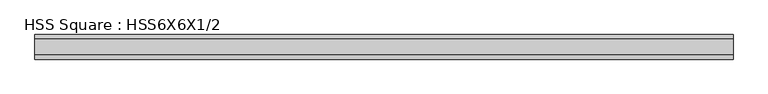
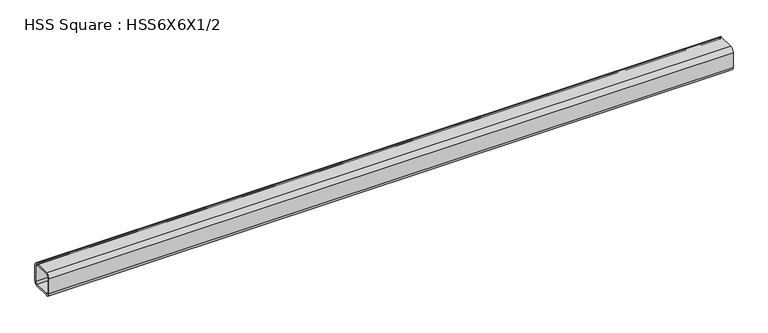
"""IFC4 building model written with IfcOpenShell, lengths in millimetres: member geometry, HSS Square : HSS6X6X1/2."""

from ifc_helpers import new_model, si_unit, point, frame, frame_2d, origin, place, context, project, spatial, polyline, circle_curve, trimmed, segment, composite_curve, outline, extrude, source, transform, mapped, element, save


def hss_square_hss6x6x1_2_b9926e2d(model_context):
    return source(origin(), model_context, "Body", "SweptSolid", [
        extrude(outline(composite_curve([segment(trimmed(circle_curve(frame_2d((-50.8, 50.8)), 25.4), [point((-76.2, 50.8))], [point((-50.8, 76.2))], False, "CARTESIAN"), True, "CONTINUOUS"), segment(polyline([(-50.8, 76.2), (50.8, 76.2)]), True, "CONTINUOUS"), segment(trimmed(circle_curve(frame_2d((50.8, 50.8)), 25.4), [point((50.8, 76.2))], [point((76.2, 50.8))], False, "CARTESIAN"), True, "CONTINUOUS"), segment(polyline([(76.2, 50.8), (76.2, -50.8)]), True, "CONTINUOUS"), segment(trimmed(circle_curve(frame_2d((50.8, -50.8)), 25.4), [point((76.2, -50.8))], [point((50.8, -76.2))], False, "CARTESIAN"), True, "CONTINUOUS"), segment(polyline([(50.8, -76.2), (-50.8, -76.2)]), True, "CONTINUOUS"), segment(trimmed(circle_curve(frame_2d((-50.8, -50.8)), 25.4), [point((-50.8, -76.2))], [point((-76.2, -50.8))], False, "CARTESIAN"), True, "CONTINUOUS"), segment(polyline([(-76.2, -50.8), (-76.2, 50.8)]), True, "CONTINUOUS")], self_intersect=False), holes=[composite_curve([segment(polyline([(50.8, 63.5), (-50.8, 63.5)]), True, "CONTINUOUS"), segment(trimmed(circle_curve(frame_2d((-50.8, 50.8)), 12.7), [point((-50.8, 63.5))], [point((-63.5, 50.8))], True, "CARTESIAN"), True, "CONTINUOUS"), segment(polyline([(-63.5, 50.8), (-63.5, -50.8)]), True, "CONTINUOUS"), segment(trimmed(circle_curve(frame_2d((-50.8, -50.8)), 12.7), [point((-63.5, -50.8))], [point((-50.8, -63.5))], True, "CARTESIAN"), True, "CONTINUOUS"), segment(polyline([(-50.8, -63.5), (50.8, -63.5)]), True, "CONTINUOUS"), segment(trimmed(circle_curve(frame_2d((50.8, -50.8)), 12.7), [point((50.8, -63.5))], [point((63.5, -50.8))], True, "CARTESIAN"), True, "CONTINUOUS"), segment(polyline([(63.5, -50.8), (63.5, 50.8)]), True, "CONTINUOUS"), segment(trimmed(circle_curve(frame_2d((50.8, 50.8)), 12.7), [point((63.5, 50.8))], [point((50.8, 63.5))], True, "CARTESIAN"), True, "CONTINUOUS")], self_intersect=False)]), frame((-2097.5113984, 0.0, 0.0), z_axis=(1.0, 0.0, 0.0), x_axis=(0.0, 1.0, 0.0)), (0.0, 0.0, 1.0), 4321.0754934),
    ])


if __name__ == "__main__":
    model = new_model("IFC4")
    model_context = context("Model", 3, world=origin())
    ifc_project = project(units=[si_unit("LENGTHUNIT", "METRE", prefix="MILLI")], contexts=[model_context])
    site = spatial("IfcSite", under=ifc_project)
    building = spatial("IfcBuilding", under=site)
    placement = place(None, origin())
    hss_square_hss6x6x1_2_shape = hss_square_hss6x6x1_2_b9926e2d(model_context)
    element("IfcMember", 1, ObjectType="HSS Square : HSS6X6X1/2", at=placement, inside=building, context=model_context, shape_type="MappedRepresentation", body=[
        mapped(hss_square_hss6x6x1_2_shape, transform((0.0, 0.0, 0.0), x_axis=(1.0, 0.0, 0.0), y_axis=(0.0, 1.0, 0.0), z_axis=(0.0, 0.0, 1.0))),
    ])
    save(model, "model.ifc")

# Revit data of these elements
# Type "HSS Square : HSS6X6X1/2"
#   Section Name Key = "HSS 6X6X1/2"
#   Assembly Code = "B10"
#   Width = 6.000"
#   Wall Nominal Thickness = 0.500"
#   Wall Design Thickness = 0.465"
#   Torsional Moment of Inertia = 81.10 in⁴
#   Torsional Modulus = 28.10 in³
#   Section Area = 9.74 in²
#   Plastic Modulus weak axis = 19.80 in³
#   Plastic Modulus strong axis = 19.80 in³
#   Outer Fillet = 1.000"
#   Nominal Weight = 35.24 lbf/ft
#   Moment of Inertia weak axis = 48.30 in⁴
#   Moment of Inertia strong axis = 48.30 in⁴
#   Inner Fillet = 0.500"
#   Height = 6.000"
#   Elastic Modulus weak axis = 16.10 in³
#   Elastic Modulus strong axis = 16.10 in³
#   Centroid Vertical = 3.000"
#   Centroid Horizontal = 3.000"
#   Length [instance default] = 5' - 0"
#   Structural Material [instance default] = Steel ASTM A500, Grade B, Rectangular and Square
#   Principal Axes Angle = 0
# Element 1 (IfcMember, "HSS Square : HSS6X6X1/2")
#   Structural Material = Steel ASTM A992
#   Materials on its faces: "Steel ASTM A992"
# Materials
#   "Steel ASTM A500, Grade B, Rectangular and Square": class "Metal", colour RGB 199 199 199, transparency 0, Description = "Carbon steel", Cost = 0
#   "Steel ASTM A992": class "Metal", colour RGB 199 199 199, transparency 0, Description = "Structural steel 50ksi", Cost = 0
